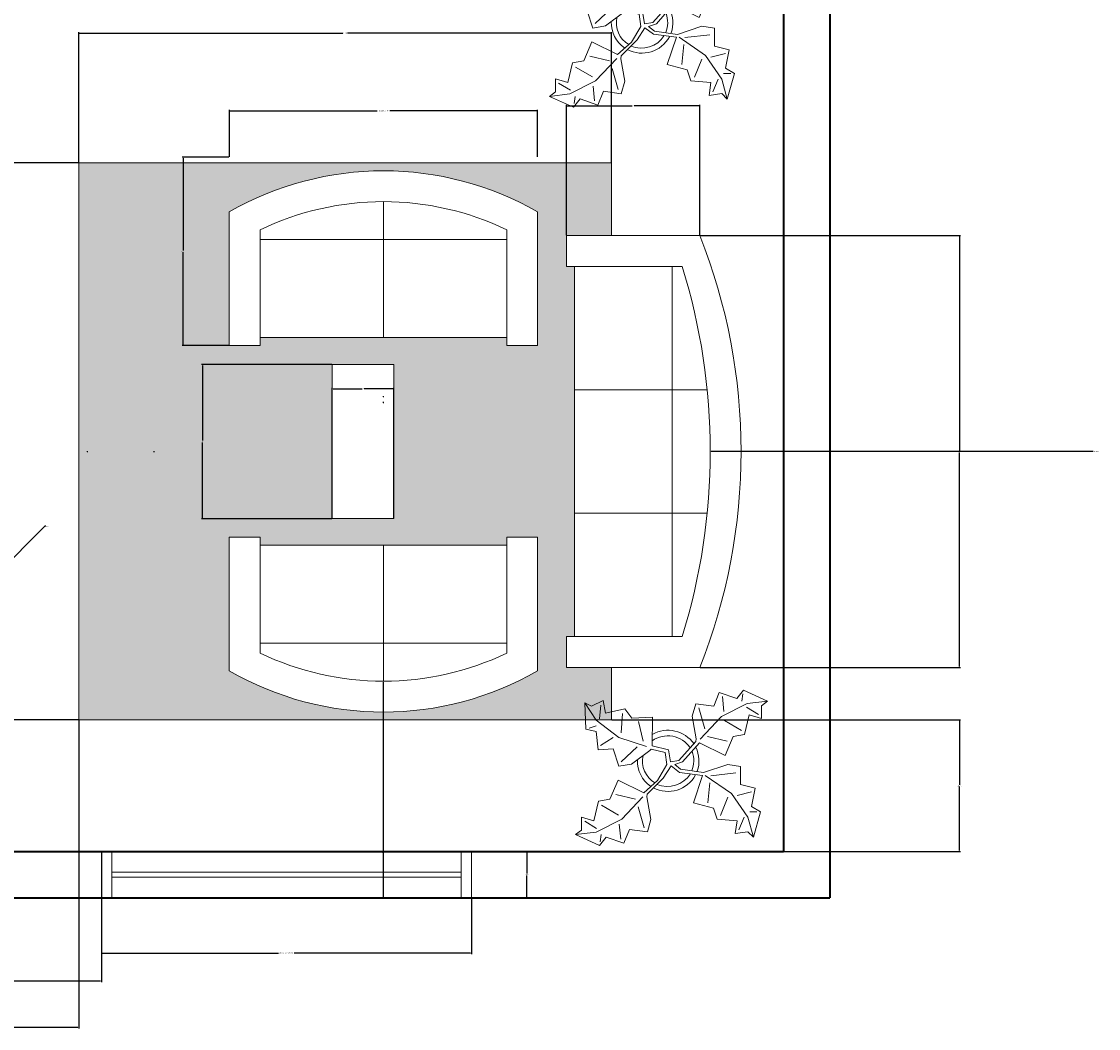
# Model space of a CAD drawing. Units: inches. Extents: x -1 to 436, y -13 to 497.
# Tile 2 of 4: x 227 to 436, y -13 to 183. Entities that reach past the tile are written whole.
import ezdxf

# ---------------------------------------------------------------- set-up
doc = ezdxf.new("R2010")
doc.units = ezdxf.units.IN
for name, color, linetype, lineweight in [('A-ANNO-DIMS', 2, 'Continuous', 18), ('A-FLOR-PATT', 9, 'Continuous', 13), ('A-FURN', 8, 'Continuous', 18), ('A-GLAZ', 4, 'Continuous', 18), ('A-PLNT', 3, 'Continuous', 13), ('A-WALL', 7, 'Continuous', 35)]:
    doc.layers.add(name, color=color, linetype=linetype, lineweight=lineweight)
doc.styles.get("Standard").update_dxf_attribs({"font": 'arial.ttf'})
doc.dimstyles.get("Standard").update_dxf_attribs({"dimtxt": 0.18, "dimasz": 0.18, "dimexe": 0.18, "dimexo": 0.0625, "dimgap": 0.09, "dimtad": 0, "dimtih": 1, "dimtoh": 1, "dimdec": 4, "dimzin": 0, "dimdsep": 46, "dimtxsty": 'Standard', "dimcen": 0.09, "dimadec": 0, "dimazin": 0, "dimtfac": 1, "dimtdec": 4, "dimtofl": 0, "dimtmove": 0, "dimatfit": 3, "dimfxl": 1, "dimtolj": 1, "dimtzin": 0, "dimarcsym": 0})

# ---------------------------------------------------------------- blocks, each defined once
blk = doc.blocks.new('Plant - Rubber or Philodendron')
for p, q in [((8.8871, 10.7908), (9.9809, 13.4933)), ((9.9809, 13.4933), (13.3837, 12.301)), ((10.5828, 12.6946), (10.8893, 9.7953)), ((13.3837, 12.301), (14.68, 13.9039)), ((14.5816, 13.2037), (14.3848, 11.8033)), ((14.68, 13.9039), (19.3848, 11.8146)), ((-16.2005, 11.4774), (-13.9899, 8.1064)), ((-16.2005, 11.4774), (-14.8639, 10.7964)), ((-16.0159, 6.3329), (-16.2005, 11.4774)), ((-14.8639, 10.7964), (-12.6195, 11.8975)), ((-13.3174, 8.325), (-13.0735, 11.0065)), ((-12.6195, 11.8975), (-12.1909, 9.4345)), ((4.6914, 8.8812), (5.3859, 11.2828)), ((5.3859, 11.2828), (8.8871, 10.7908)), ((5.9878, 10.4842), (7.1971, 6.3869)), ((15.3859, 11.3055), (10.3916, 8.7942)), ((15.2875, 10.6053), (17.5907, 9.2105)), ((19.3848, 11.8146), (15.3859, 11.3055)), ((19.3848, 11.8146), (18.1868, 10.9119)), ((18.1868, 10.9119), (18.1925, 8.4119)), ((-12.1909, 9.4345), (-8.3829, 10.3)), ((-8.8369, 9.409), (-9.0894, 5.6095)), ((-8.3829, 10.3), (-7.0549, 8.501)), ((-7.0549, 8.501), (-3.0284, 8.6941)), ((-3.0284, 8.6941), (-3.0709, 3.1041)), ((4.6914, 8.8812), (5.5014, 4.4831)), ((10.3916, 8.7942), (6.2847, 4.4028)), ((15.7909, 9.1065), (14.8995, 5.3044)), ((18.1925, 8.4119), (15.7909, 9.1065)), ((-14.0069, 5.8704), (-16.0159, 6.3329)), ((-15.3434, 6.5514), (-13.9984, 6.9884)), ((-13.9899, 8.1064), (-9.5434, 4.7185)), ((-4.8529, 4.012), (-5.7184, 7.82)), ((14.2977, 6.1031), (10.9934, 7.9956)), ((-13.5868, 2.2894), (-14.0069, 5.8704)), ((-13.1329, 3.1804), (-10.6614, 4.727)), ((-9.5434, 4.7185), (-4.1917, 2.9888)), ((5.4346, 3.9146), (5.5014, 4.4831)), ((7.7005, 4.8881), (11.5025, 3.9967)), ((12.7005, 4.8994), (11.1089, 1.1958)), ((14.8995, 5.3044), (12.7005, 4.8994)), ((-10.6784, 2.491), (-13.5868, 2.2894)), ((-9.5858, -0.8715), (-10.6784, 2.491)), ((-9.1318, 0.0195), (-5.9793, 2.9025)), ((-7.1228, -0.443), (-3.5248, 2.2131)), ((-3.5248, 2.2131), (-3.3011, 2.4355)), ((-3.3011, 2.4355), (-0.5306, 1.7947)), ((-3.0709, 3.1041), (0.0797, 2.3163)), ((0.0797, 2.3163), (0.4866, -0.031)), ((2.1141, 0.2298), (5.4346, 3.9146)), ((6.1032, 3.6844), (2.8262, -0.031)), ((11.1089, 1.1958), (6.1032, 3.6844)), ((-0.5306, 1.7947), (-0.2255, -0.5527)), ((-0.5306, 1.7947), (-0.5306, 1.7947)), ((0.4866, -0.031), (2.1141, 0.2298)), ((-7.1228, -0.443), (-9.5858, -0.8715)), ((-2.019, -3.6148), (-0.2255, -0.5527)), ((-0.9375, -3.1608), (0.5883, -0.8135)), ((0.5883, -0.8135), (2.2447, -2.0916)), ((2.8262, -0.031), (1.3003, -0.5527)), ((1.3003, -0.5527), (2.4193, -1.4655)), ((2.2447, -2.0916), (6.7108, -2.6626)), ((2.4193, -1.4655), (6.895, -2.1175)), ((11.6605, -0.5413), (6.895, -2.1175)), ((11.6605, -0.5413), (14.1354, -0.8948)), ((14.1354, -0.8948), (14.1354, -4.4304)), ((-11.3237, -7.2629), (-9.7321, -3.5593)), ((-9.7321, -3.5593), (-4.7264, -6.0479)), ((-2.019, -3.6148), (-4.7264, -6.0479)), ((-4.0579, -6.2781), (-0.9375, -3.1608)), ((4.943, -7.9659), (6.7108, -2.6626)), ((12.3677, -6.1981), (7.219, -2.6772)), ((8.125, -4.0768), (7.7715, -7.9659)), ((8.3544, -2.7453), (13.1973, -2.1704)), ((-4.1246, -6.8466), (-4.0579, -6.2781)), ((15.5496, -10.7943), (12.3677, -6.1981)), ((16.2567, -5.8446), (13.4283, -6.5517)), ((14.1354, -4.4304), (16.9638, -5.1375)), ((16.9638, -5.1375), (16.2567, -8.673)), ((-14.4141, -11.4699), (-13.5228, -7.6679)), ((-13.5228, -7.6679), (-11.3237, -7.2629)), ((-6.3237, -7.2516), (-10.1257, -6.3602)), ((-9.0148, -11.1577), (-4.9047, -6.8122)), ((-3.3146, -11.2447), (-4.1246, -6.8466)), ((8.8321, -9.0266), (4.943, -7.9659)), ((10.2463, -10.4408), (11.6605, -6.9053)), ((-12.921, -8.4665), (-9.6166, -10.359)), ((-4.611, -12.8477), (-5.8203, -8.7504)), ((9.5392, -11.1479), (8.8321, -9.0266)), ((17.3174, -9.7337), (15.9032, -9.7337)), ((16.2567, -8.673), (18.0245, -9.7337)), ((18.0245, -9.7337), (16.6103, -14.6834)), ((-16.8157, -10.7754), (-14.4141, -11.4699)), ((-16.8101, -13.2754), (-16.8157, -10.7754)), ((-13.9107, -12.9688), (-16.2139, -11.574)), ((-14.0091, -13.669), (-9.0148, -11.1577)), ((-9.206, -15.0581), (-9.5126, -12.1588)), ((-3.3146, -11.2447), (-4.0092, -13.6463)), ((13.4283, -11.5015), (9.5392, -11.1479)), ((13.0748, -13.9763), (13.4283, -11.5015)), ((14.8425, -10.7943), (13.7819, -13.2692)), ((16.6103, -14.6834), (15.5496, -10.7943)), ((-18.008, -14.1781), (-16.8101, -13.2754)), ((-18.008, -14.1781), (-14.0091, -13.669)), ((-13.3032, -16.2674), (-18.008, -14.1781)), ((-12.0069, -14.6645), (-13.3032, -16.2674)), ((-13.2048, -15.5672), (-13.008, -14.1668)), ((-8.6042, -15.8568), (-12.0069, -14.6645)), ((-7.5103, -13.1543), (-8.6042, -15.8568)), ((-4.0092, -13.6463), (-7.5103, -13.1543)), ((15.5496, -13.6228), (13.0748, -13.9763)), ((16.6103, -14.6834), (15.5496, -13.6228))]:
    blk.add_line(p, q)
for centre, radius, start, end in [((0, 0), 6.1275, 34.37569, 120.1028), ((-0.0601, -0.2075), 5.2461, 33.82192, 124.9414), ((-0.098, 0.1364), 6.1288, 341.2017, 26.09184), ((0.0308, 0.1664), 6, 178.6147, 235.1169), ((0.0308, 0.1664), 5, 168.1647, 238.6725), ((-0.2664, 0.1682), 5.2775, 338.4094, 20.03007), ((-0.0234, 0.3825), 6.1492, 242.5812, 331.2714), ((-0.1102, 0.4886), 5.2883, 247.3711, 327.472)]:
    blk.add_arc(centre, radius, start, end)
blk = doc.blocks.new('SOFA-LOVESEAT-60')
for p, q in [((6, 34), (6, 11.47)), ((54, 34), (54, 11.47)), ((54, 32.44), (6, 32.44)), ((30, 32.44), (30, 6)), ((54, 13.38), (6, 13.38))]:
    blk.add_line(p, q)
for points in [[(0, 8), (0, 34), (6, 34)], [(54, 34), (60, 34), (60, 8)]]:
    blk.add_lwpolyline(points)
for centre, radius, start, end in [((30, 61.38), 55.38, 244.3208, 295.6792), ((30, 60.25), 60.25, 240.1371, 299.8628)]:
    blk.add_arc(centre, radius, start, end)
blk = doc.blocks.new('WIN-FIXED-72')
for p, q in [((2, 0), (2, 9)), ((70, 0), (70, 9)), ((2, 5), (70, 5)), ((2, 4), (70, 4))]:
    blk.add_line(p, q)
blk.add_lwpolyline([(0, 9), (72, 9), (72, 0), (0, 0)], close=True)
blk = doc.blocks.new('*D20')
at = {"layer": 'A-ANNO-DIMS', "color": 0, "lineweight": -2, "transparency": 16777216}
for p, q in [((267.14, 156.67), (267.14, 165.79)), ((267.32, 165.61), (295.91, 165.61)), ((326.96, 165.61), (298.36, 165.61)), ((327.14, 156.67), (327.14, 165.79))]:
    blk.add_line(p, q, dxfattribs=at)
at = {"layer": 'A-ANNO-DIMS', "color": 0, "transparency": 16777216}
for points in [[(267.32, 165.64), (267.32, 165.58), (267.14, 165.61)], [(326.96, 165.64), (326.96, 165.58), (327.14, 165.61)]]:
    blk.add_solid(points, dxfattribs=at)
at = {"layer": 'Defpoints', "color": 0, "transparency": 16777216}
for p in [(267.14, 165.61), (267.14, 156.61), (327.14, 156.61)]:
    blk.add_point(p, dxfattribs=at)
at = {"layer": 'A-ANNO-DIMS', "color": 0, "transparency": 16777216, "insert": (297.14, 165.61), "char_height": 0.18, "attachment_point": 5}
blk.add_mtext('\\A1;LOVESEAT 60 TYP.', dxfattribs=at)
blk = doc.blocks.new('*D21')
at = {"layer": 'A-ANNO-DIMS', "color": 0, "lineweight": -2, "transparency": 16777216}
for p, q in [((267.07, 156.61), (257.96, 156.61)), ((258.14, 156.43), (258.14, 138.46)), ((258.14, 120.12), (258.14, 138.09)), ((267.07, 119.94), (257.96, 119.94))]:
    blk.add_line(p, q, dxfattribs=at)
at = {"layer": 'A-ANNO-DIMS', "color": 0, "transparency": 16777216}
for points in [[(258.11, 156.43), (258.17, 156.43), (258.14, 156.61)], [(258.11, 120.12), (258.17, 120.12), (258.14, 119.94)]]:
    blk.add_solid(points, dxfattribs=at)
at = {"layer": 'Defpoints', "color": 0, "transparency": 16777216}
for p in [(267.14, 156.61), (258.14, 119.94), (267.14, 119.94)]:
    blk.add_point(p, dxfattribs=at)
at = {"layer": 'A-ANNO-DIMS', "color": 0, "transparency": 16777216, "insert": (258.14, 138.28), "char_height": 0.18, "attachment_point": 5}
blk.add_mtext('\\A1;37 TYP.', dxfattribs=at)
blk = doc.blocks.new('*D22')
at = {"layer": 'A-ANNO-DIMS', "color": 0, "lineweight": -2, "transparency": 16777216}
for p, q in [((242.25, 12.47), (242.25, 1.55)), ((314.25, 12.47), (314.25, 1.55)), ((242.43, 1.73), (276.74, 1.73)), ((314.07, 1.73), (279.76, 1.73))]:
    blk.add_line(p, q, dxfattribs=at)
at = {"layer": 'A-ANNO-DIMS', "color": 0, "transparency": 16777216}
for points in [[(242.43, 1.76), (242.43, 1.7), (242.25, 1.73)], [(314.07, 1.76), (314.07, 1.7), (314.25, 1.73)]]:
    blk.add_solid(points, dxfattribs=at)
at = {"layer": 'Defpoints', "color": 0, "transparency": 16777216}
for p in [(242.25, 12.53), (314.25, 12.53), (314.25, 1.73)]:
    blk.add_point(p, dxfattribs=at)
at = {"layer": 'A-ANNO-DIMS', "color": 0, "transparency": 16777216, "insert": (278.25, 1.73), "char_height": 0.18, "attachment_point": 5}
blk.add_mtext('\\A1;FIXED WINDOW 72 TYP.', dxfattribs=at)
blk = doc.blocks.new('*D23')
at = {"layer": 'A-ANNO-DIMS', "color": 0, "lineweight": -2, "transparency": 16777216}
for p, q in [((314.31, 21.53), (325.23, 21.53)), ((325.05, 21.35), (325.05, 17.22)), ((325.05, 12.71), (325.05, 16.85)), ((314.31, 12.53), (325.23, 12.53))]:
    blk.add_line(p, q, dxfattribs=at)
at = {"layer": 'A-ANNO-DIMS', "color": 0, "transparency": 16777216}
for points in [[(325.02, 21.35), (325.08, 21.35), (325.05, 21.53)], [(325.02, 12.71), (325.08, 12.71), (325.05, 12.53)]]:
    blk.add_solid(points, dxfattribs=at)
at = {"layer": 'Defpoints', "color": 0, "transparency": 16777216}
for p in [(314.25, 21.53), (325.05, 21.53), (314.25, 12.53)]:
    blk.add_point(p, dxfattribs=at)
at = {"layer": 'A-ANNO-DIMS', "color": 0, "transparency": 16777216, "insert": (325.05, 17.03), "char_height": 0.18, "attachment_point": 5}
blk.add_mtext('\\A1;9 TYP.', dxfattribs=at)
blk = doc.blocks.new('*D30')
at = {"layer": 'A-ANNO-DIMS', "color": 0, "lineweight": -2, "transparency": 16777216}
for p, q in [((181.5, 21.47), (181.5, -3.9)), ((242.25, 21.47), (242.25, -3.9)), ((181.68, -3.72), (211.48, -3.72)), ((242.07, -3.72), (212.27, -3.72))]:
    blk.add_line(p, q, dxfattribs=at)
at = {"layer": 'A-ANNO-DIMS', "color": 0, "transparency": 16777216}
for points in [[(181.68, -3.69), (181.68, -3.75), (181.5, -3.72)], [(242.07, -3.69), (242.07, -3.75), (242.25, -3.72)]]:
    blk.add_solid(points, dxfattribs=at)
at = {"layer": 'Defpoints', "color": 0, "transparency": 16777216}
for p in [(181.5, 21.53), (242.25, 21.53), (181.5, -3.72)]:
    blk.add_point(p, dxfattribs=at)
at = {"layer": 'A-ANNO-DIMS', "color": 0, "transparency": 16777216, "insert": (211.88, -3.72), "char_height": 0.18, "attachment_point": 5}
blk.add_mtext('\\A1;60.75', dxfattribs=at)
blk = doc.blocks.new('*D66')
at = {"layer": 'A-ANNO-DIMS', "color": 0, "lineweight": -2, "transparency": 16777216}
for p, q in [((287.11, 116.27), (261.74, 116.27)), ((261.92, 116.09), (261.92, 101.46)), ((261.92, 86.45), (261.92, 101.09)), ((287.11, 86.27), (261.74, 86.27))]:
    blk.add_line(p, q, dxfattribs=at)
at = {"layer": 'A-ANNO-DIMS', "color": 0, "transparency": 16777216}
for points in [[(261.89, 116.09), (261.95, 116.09), (261.92, 116.27)], [(261.89, 86.45), (261.95, 86.45), (261.92, 86.27)]]:
    blk.add_solid(points, dxfattribs=at)
at = {"layer": 'Defpoints', "color": 0, "transparency": 16777216}
for p in [(261.92, 116.27), (287.17, 116.27), (287.17, 86.27)]:
    blk.add_point(p, dxfattribs=at)
at = {"layer": 'A-ANNO-DIMS', "color": 0, "transparency": 16777216, "insert": (261.92, 101.27), "char_height": 0.18, "attachment_point": 5}
blk.add_mtext('\\A1;30', dxfattribs=at)
blk = doc.blocks.new('*D67')
at = {"layer": 'A-ANNO-DIMS', "color": 0, "lineweight": -2, "transparency": 16777216}
for p, q in [((287.17, 86.34), (287.17, 111.7)), ((287.35, 111.52), (292.97, 111.52)), ((298.99, 111.52), (293.38, 111.52)), ((299.17, 86.34), (299.17, 111.7))]:
    blk.add_line(p, q, dxfattribs=at)
at = {"layer": 'A-ANNO-DIMS', "color": 0, "transparency": 16777216}
for points in [[(287.35, 111.55), (287.35, 111.49), (287.17, 111.52)], [(298.99, 111.55), (298.99, 111.49), (299.17, 111.52)]]:
    blk.add_solid(points, dxfattribs=at)
at = {"layer": 'Defpoints', "color": 0, "transparency": 16777216}
for p in [(299.17, 111.52), (287.17, 86.27), (299.17, 86.27)]:
    blk.add_point(p, dxfattribs=at)
at = {"layer": 'A-ANNO-DIMS', "color": 0, "transparency": 16777216, "insert": (293.17, 111.52), "char_height": 0.18, "attachment_point": 5}
blk.add_mtext('\\A1;12', dxfattribs=at)
blk = doc.blocks.new('*D68')
at = {"layer": 'A-ANNO-DIMS', "color": 0, "lineweight": -2, "transparency": 16777216}
for p, q in [((358.8, 141.33), (409.43, 141.33)), ((409.25, 141.15), (409.25, 99.51)), ((409.25, 57.51), (409.25, 99.15)), ((358.8, 57.33), (409.43, 57.33))]:
    blk.add_line(p, q, dxfattribs=at)
at = {"layer": 'A-ANNO-DIMS', "color": 0, "transparency": 16777216}
for points in [[(409.22, 141.15), (409.28, 141.15), (409.25, 141.33)], [(409.22, 57.51), (409.28, 57.51), (409.25, 57.33)]]:
    blk.add_solid(points, dxfattribs=at)
at = {"layer": 'Defpoints', "color": 0, "transparency": 16777216}
for p in [(358.74, 141.33), (358.74, 57.33), (409.25, 57.33)]:
    blk.add_point(p, dxfattribs=at)
at = {"layer": 'A-ANNO-DIMS', "color": 0, "transparency": 16777216, "insert": (409.25, 99.33), "char_height": 0.18, "attachment_point": 5}
blk.add_mtext('\\A1;84', dxfattribs=at)
blk = doc.blocks.new('*D69')
at = {"layer": 'A-ANNO-DIMS', "color": 0, "lineweight": -2, "transparency": 16777216}
for p, q in [((332.74, 141.39), (332.74, 166.76)), ((332.92, 166.58), (345.51, 166.58)), ((358.56, 166.58), (345.96, 166.58)), ((358.74, 141.39), (358.74, 166.76))]:
    blk.add_line(p, q, dxfattribs=at)
at = {"layer": 'A-ANNO-DIMS', "color": 0, "transparency": 16777216}
for points in [[(332.92, 166.61), (332.92, 166.55), (332.74, 166.58)], [(358.56, 166.61), (358.56, 166.55), (358.74, 166.58)]]:
    blk.add_solid(points, dxfattribs=at)
at = {"layer": 'Defpoints', "color": 0, "transparency": 16777216}
for p in [(358.74, 166.58), (332.74, 141.33), (358.74, 141.33)]:
    blk.add_point(p, dxfattribs=at)
at = {"layer": 'A-ANNO-DIMS', "color": 0, "transparency": 16777216, "insert": (345.74, 166.58), "char_height": 0.18, "attachment_point": 5}
blk.add_mtext('\\A1;26', dxfattribs=at)
blk = doc.blocks.new('*D70')
at = {"layer": 'A-ANNO-DIMS', "color": 0, "lineweight": -2, "transparency": 16777216}
for p, q in [((237.77, 155.49), (212.4, 155.49)), ((212.58, 155.31), (212.58, 101.48)), ((212.58, 47.29), (212.58, 101.11)), ((237.77, 47.11), (212.4, 47.11))]:
    blk.add_line(p, q, dxfattribs=at)
at = {"layer": 'A-ANNO-DIMS', "color": 0, "transparency": 16777216}
for points in [[(212.55, 155.31), (212.61, 155.31), (212.58, 155.49)], [(212.55, 47.29), (212.61, 47.29), (212.58, 47.11)]]:
    blk.add_solid(points, dxfattribs=at)
at = {"layer": 'Defpoints', "color": 0, "transparency": 16777216}
for p in [(212.58, 155.49), (237.83, 155.49), (237.83, 47.11)]:
    blk.add_point(p, dxfattribs=at)
at = {"layer": 'A-ANNO-DIMS', "color": 0, "transparency": 16777216, "insert": (212.58, 101.3), "char_height": 0.18, "attachment_point": 5}
blk.add_mtext('\\A1;108.38', dxfattribs=at)
blk = doc.blocks.new('*D71')
at = {"layer": 'A-ANNO-DIMS', "color": 0, "lineweight": -2, "transparency": 16777216}
for p, q in [((237.83, 155.55), (237.83, 180.92)), ((238.01, 180.74), (289.21, 180.74)), ((341.33, 180.74), (290.12, 180.74)), ((341.51, 155.55), (341.51, 180.92))]:
    blk.add_line(p, q, dxfattribs=at)
at = {"layer": 'A-ANNO-DIMS', "color": 0, "transparency": 16777216}
for points in [[(238.01, 180.77), (238.01, 180.71), (237.83, 180.74)], [(341.33, 180.77), (341.33, 180.71), (341.51, 180.74)]]:
    blk.add_solid(points, dxfattribs=at)
at = {"layer": 'Defpoints', "color": 0, "transparency": 16777216}
for p in [(341.51, 180.74), (237.83, 155.49), (341.51, 155.49)]:
    blk.add_point(p, dxfattribs=at)
at = {"layer": 'A-ANNO-DIMS', "color": 0, "transparency": 16777216, "insert": (289.67, 180.74), "char_height": 0.18, "attachment_point": 5}
blk.add_mtext('\\A1;103.68', dxfattribs=at)
blk = doc.blocks.new('*D72')
at = {"layer": 'A-ANNO-DIMS', "color": 0, "lineweight": -2, "transparency": 16777216}
for p, q in [((237.83, 229.51), (212.46, 229.53)), ((212.64, 229.35), (212.61, 192.7)), ((212.58, 155.69), (212.61, 192.34)), ((237.77, 155.49), (212.4, 155.51))]:
    blk.add_line(p, q, dxfattribs=at)
at = {"layer": 'A-ANNO-DIMS', "color": 0, "transparency": 16777216}
for points in [[(212.61, 229.35), (212.67, 229.35), (212.64, 229.53)], [(212.55, 155.69), (212.61, 155.69), (212.58, 155.51)]]:
    blk.add_solid(points, dxfattribs=at)
at = {"layer": 'Defpoints', "color": 0, "transparency": 16777216}
for p in [(212.64, 229.53), (237.89, 229.51), (237.83, 155.49)]:
    blk.add_point(p, dxfattribs=at)
at = {"layer": 'A-ANNO-DIMS', "color": 0, "transparency": 16777216, "insert": (212.61, 192.52), "char_height": 0.18, "attachment_point": 5}
blk.add_mtext('\\A1;74.03', dxfattribs=at)
blk = doc.blocks.new('*D76')
at = {"layer": 'A-ANNO-DIMS', "color": 0, "lineweight": -2, "transparency": 16777216}
for p, q in [((341.57, 47.11), (409.43, 47.11)), ((409.25, 46.93), (409.25, 34.5)), ((409.25, 21.71), (409.25, 34.14)), ((375.06, 21.53), (409.43, 21.53))]:
    blk.add_line(p, q, dxfattribs=at)
at = {"layer": 'A-ANNO-DIMS', "color": 0, "transparency": 16777216}
for points in [[(409.22, 46.93), (409.28, 46.93), (409.25, 47.11)], [(409.22, 21.71), (409.28, 21.71), (409.25, 21.53)]]:
    blk.add_solid(points, dxfattribs=at)
at = {"layer": 'Defpoints', "color": 0, "transparency": 16777216}
for p in [(341.51, 47.11), (409.25, 47.11), (375, 21.53)]:
    blk.add_point(p, dxfattribs=at)
at = {"layer": 'A-ANNO-DIMS', "color": 0, "transparency": 16777216, "insert": (409.25, 34.32), "char_height": 0.18, "attachment_point": 5}
blk.add_mtext('\\A1;25.573', dxfattribs=at)
blk = doc.blocks.new('*D77')
at = {"layer": 'A-ANNO-DIMS', "color": 0, "lineweight": -2, "transparency": 16777216}
for p, q in [((237.83, 47.04), (237.83, -12.9)), ((181.5, 21.47), (181.5, -12.9)), ((181.68, -12.72), (209.27, -12.72)), ((237.65, -12.72), (210.06, -12.72))]:
    blk.add_line(p, q, dxfattribs=at)
at = {"layer": 'A-ANNO-DIMS', "color": 0, "transparency": 16777216}
for points in [[(181.68, -12.69), (181.68, -12.75), (181.5, -12.72)], [(237.65, -12.69), (237.65, -12.75), (237.83, -12.72)]]:
    blk.add_solid(points, dxfattribs=at)
at = {"layer": 'Defpoints', "color": 0, "transparency": 16777216}
for p in [(237.83, 47.11), (181.5, 21.53), (237.83, -12.72)]:
    blk.add_point(p, dxfattribs=at)
at = {"layer": 'A-ANNO-DIMS', "color": 0, "transparency": 16777216, "insert": (209.67, -12.72), "char_height": 0.18, "attachment_point": 5}
blk.add_mtext('\\A1;56.33', dxfattribs=at)
blk = doc.blocks.new('*D78')
at = {"layer": 'A-ANNO-DIMS', "color": 0, "lineweight": -2, "transparency": 16777216}
for p, q in [((252.4, 99.33), (252.58, 99.33)), ((252.49, 99.24), (252.49, 99.42)), ((435.29, 99.33), (366.92, 99.33))]:
    blk.add_line(p, q, dxfattribs=at)
at = {"layer": 'A-ANNO-DIMS', "color": 0, "transparency": 16777216}
blk.add_solid([(366.92, 99.36), (366.92, 99.3), (366.74, 99.33)], dxfattribs=at)
at = {"layer": 'Defpoints', "color": 0, "transparency": 16777216}
for p in [(252.49, 99.33), (366.74, 99.33)]:
    blk.add_point(p, dxfattribs=at)
at = {"layer": 'A-ANNO-DIMS', "color": 0, "transparency": 16777216, "insert": (435.84, 99.33), "char_height": 0.18, "attachment_point": 5}
blk.add_mtext('\\A1;R114.25', dxfattribs=at)
blk = doc.blocks.new('*D79')
at = {"layer": 'A-ANNO-DIMS', "color": 0, "lineweight": -2, "transparency": 16777216}
for p, q in [((239.45, 99.33), (239.63, 99.33)), ((239.54, 99.24), (239.54, 99.42)), ((433.45, 99.33), (360.92, 99.33))]:
    blk.add_line(p, q, dxfattribs=at)
at = {"layer": 'A-ANNO-DIMS', "color": 0, "transparency": 16777216}
blk.add_solid([(360.92, 99.36), (360.92, 99.3), (360.74, 99.33)], dxfattribs=at)
at = {"layer": 'Defpoints', "color": 0, "transparency": 16777216}
for p in [(239.54, 99.33), (360.74, 99.33)]:
    blk.add_point(p, dxfattribs=at)
at = {"layer": 'A-ANNO-DIMS', "color": 0, "transparency": 16777216, "insert": (433.93, 99.33), "char_height": 0.18, "attachment_point": 5}
blk.add_mtext('\\A1;R121.2', dxfattribs=at)
blk = doc.blocks.new('*D80')
at = {"layer": 'A-ANNO-DIMS', "color": 0, "lineweight": -2, "transparency": 16777216}
for p, q in [((297.14, 108.81), (297.14, 108.99)), ((297.05, 108.9), (297.23, 108.9)), ((297.13, 12.5), (297.13, 48.47)), ((296.95, 12.5), (297.13, 12.5))]:
    blk.add_line(p, q, dxfattribs=at)
at = {"layer": 'A-ANNO-DIMS', "color": 0, "transparency": 16777216}
blk.add_solid([(297.1, 48.47), (297.16, 48.47), (297.13, 48.65)], dxfattribs=at)
at = {"layer": 'Defpoints', "color": 0, "transparency": 16777216}
for p in [(297.14, 108.9), (297.13, 48.65)]:
    blk.add_point(p, dxfattribs=at)
at = {"layer": 'A-ANNO-DIMS', "color": 0, "transparency": 16777216, "insert": (296.28, 12.5), "char_height": 0.18, "attachment_point": 5}
blk.add_mtext('\\A1;2X R60.25', dxfattribs=at)
blk = doc.blocks.new('*D81')
at = {"layer": 'A-ANNO-DIMS', "color": 0, "lineweight": -2, "transparency": 16777216}
for p, q in [((297.05, 110.04), (297.23, 110.04)), ((297.14, 109.95), (297.14, 110.13)), ((297.13, 21.42), (297.13, 54.47)), ((296.95, 21.42), (297.13, 21.42))]:
    blk.add_line(p, q, dxfattribs=at)
at = {"layer": 'A-ANNO-DIMS', "color": 0, "transparency": 16777216}
blk.add_solid([(297.1, 54.47), (297.16, 54.47), (297.13, 54.65)], dxfattribs=at)
at = {"layer": 'Defpoints', "color": 0, "transparency": 16777216}
for p in [(297.14, 110.04), (297.13, 54.65)]:
    blk.add_point(p, dxfattribs=at)
at = {"layer": 'A-ANNO-DIMS', "color": 0, "transparency": 16777216, "insert": (296.28, 21.42), "char_height": 0.18, "attachment_point": 5}
blk.add_mtext('\\A1;2X R55.38', dxfattribs=at)
blk = doc.blocks.new('*D83')
at = {"layer": 'A-ANNO-DIMS', "color": 0, "lineweight": -2, "transparency": 16777216}
for p, q in [((231.24, 84.78), (211.22, 64.75)), ((231.42, 84.78), (231.24, 84.78)), ((177.41, 31.03), (177.59, 31.03)), ((177.5, 30.94), (177.5, 31.12))]:
    blk.add_line(p, q, dxfattribs=at)
at = {"layer": 'A-ANNO-DIMS', "color": 0, "transparency": 16777216}
blk.add_solid([(211.2, 64.77), (211.24, 64.73), (211.09, 64.62)], dxfattribs=at)
at = {"layer": 'Defpoints', "color": 0, "transparency": 16777216}
for p in [(211.09, 64.62), (177.5, 31.03)]:
    blk.add_point(p, dxfattribs=at)
at = {"layer": 'A-ANNO-DIMS', "color": 0, "transparency": 16777216, "insert": (231.83, 84.78), "char_height": 0.18, "attachment_point": 5}
blk.add_mtext('\\A1;R47.5', dxfattribs=at)

msp = doc.modelspace()

# ---------------------------------------------------------------- hatches: boundary and pattern name
at = {"layer": 'A-FLOR-PATT'}
h = msp.add_hatch(color=256, dxfattribs=at)
h.dxf.hatch_style = 1
h.paths.add_polyline_path([(334.2932, 135.3315), (332.7353, 135.3315), (332.7353, 141.3315), (341.5066, 141.3315), (341.5066, 155.4864), (237.8302, 155.4864), (237.8302, 47.1064), (341.5066, 47.1064), (341.5066, 57.3315), (332.7353, 57.3315), (332.7353, 63.3315), (334.2932, 63.3315)])
h.paths.add_polyline_path([(321.1354, 119.9418), (321.1354, 121.4998), (273.1354, 121.4998), (273.1354, 119.9418), (267.1354, 119.9418), (267.1354, 145.9417, -0.26666697), (327.1354, 145.9417), (327.1354, 119.9418)], flags=16)
h.paths.add_polyline_path([(299.175, 86.2737), (287.175, 86.2737), (287.175, 116.2737), (299.175, 116.2737)], flags=16)
h.paths.add_polyline_path([(321.1354, 82.6511), (327.1354, 82.6511), (327.1354, 56.6511, -0.26666697), (267.1354, 56.6511), (267.1354, 82.6511), (273.1354, 82.6511), (273.1354, 81.0931), (321.1354, 81.0931)], flags=16)

# ---------------------------------------------------------------- linework, layer by layer
at = {"layer": 'A-FURN'}
for p, q in [((237.8302, 155.4864), (341.5066, 155.4864)), ((237.8302, 47.1064), (237.8302, 155.4864)), ((341.5066, 155.4864), (341.5066, 141.3315)), ((332.7353, 135.3315), (355.2657, 135.3315)), ((334.2932, 135.3315), (334.2932, 63.3315)), ((353.3534, 135.3313), (353.3534, 63.3317)), ((299.175, 116.2737), (287.175, 116.2737)), ((287.175, 116.2737), (287.175, 86.2737)), ((299.175, 86.2737), (299.175, 116.2737)), ((334.2932, 111.3315), (360.1382, 111.3315)), ((287.175, 86.2737), (299.175, 86.2737)), ((334.2932, 87.3315), (360.1382, 87.3315)), ((332.7353, 63.3315), (355.2657, 63.3315)), ((341.5066, 57.3315), (341.5066, 47.1064)), ((341.5066, 47.1064), (237.8302, 47.1064))]:
    msp.add_line(p, q, dxfattribs=at)
for points in [[(332.7353, 135.3315), (332.7353, 141.3315), (358.7353, 141.3315)], [(358.7353, 57.3315), (332.7353, 57.3315), (332.7353, 63.3315)]]:
    msp.add_lwpolyline(points, dxfattribs=at)
for centre, radius, start, end in [((252.4853, 99.3315), 114.25, 338.43141, 21.5686), ((239.5385, 99.3315), 121.1968, 342.72033, 17.2797)]:
    msp.add_arc(centre, radius, start, end, dxfattribs=at)
at = {"layer": 'A-WALL'}
for p, q in [((384, 471.5331), (384, 12.5331)), ((375, 390.5331), (375, 21.5331)), ((181.5, 21.5331), (375, 21.5331)), ((177, 12.5331), (384, 12.5331))]:
    msp.add_line(p, q, dxfattribs=at)

# ---------------------------------------------------------------- block references
at = {"layer": 'A-FURN', "rotation": 180.0000448048175}
msp.add_blockref('SOFA-LOVESEAT-60', (327.1358, 153.9419), dxfattribs=at)
at = {"layer": 'A-FURN'}
msp.add_blockref('SOFA-LOVESEAT-60', (267.135, 48.651), dxfattribs=at)
at = {"layer": 'A-GLAZ'}
msp.add_blockref('WIN-FIXED-72', (242.25, 12.533), dxfattribs=at)
at = {"layer": 'A-PLNT'}
for p in [(347.4393, 182.5896), (352.5154, 38.9808)]:
    msp.add_blockref('Plant - Rubber or Philodendron', p, dxfattribs=at)

# ---------------------------------------------------------------- dimensions: what is measured, and where the dimension line sits
at = {"layer": 'A-ANNO-DIMS'}
for base, p1, p2, angle, override, picture, middle in [((212.6448, 229.5338), (237.8302, 155.4864), (237.8948, 229.5117), 89.949986, {"dimdec": 2, "dimlfac": 1, "dimrnd": 0, "dimzin": 0, "dimdsep": 46, "dimlunit": 2}, '*D72', (212.6125, 192.5211)), ((358.7353, 166.5815), (332.7353, 141.3315), (358.7353, 141.3315), 359.999958, {"dimdec": 0, "dimlfac": 1, "dimrnd": 0, "dimzin": 0, "dimdsep": 46, "dimlunit": 2}, '*D69', (345.7353, 166.5815)), ((212.5802, 155.4864), (237.8302, 47.1064), (237.8302, 155.4864), 90, {"dimdec": 2, "dimlfac": 1, "dimrnd": 0, "dimzin": 0, "dimdsep": 46, "dimlunit": 2}, '*D70', (212.5802, 101.2964)), ((409.25, 57.3315), (358.7353, 141.3315), (358.7353, 57.3315), 90, {"dimdec": 0, "dimlfac": 1, "dimrnd": 0, "dimzin": 0, "dimdsep": 46, "dimlunit": 2}, '*D68', (409.25, 99.3315)), ((261.925, 116.2737), (287.175, 86.2737), (287.175, 116.2737), 90, {"dimdec": 0, "dimlfac": 1, "dimrnd": 0, "dimzin": 0, "dimdsep": 46, "dimlunit": 2}, '*D66', (261.925, 101.2737)), ((409.25, 47.1064), (375, 21.5331), (341.5066, 47.1064), 90, {"dimdec": 3, "dimlfac": 1, "dimrnd": 0, "dimzin": 0, "dimdsep": 46, "dimlunit": 2}, '*D76', (409.25, 34.3198)), ((181.5, -3.7169), (242.25, 21.5331), (181.5, 21.5331), 180, {"dimdec": 2, "dimlfac": 1, "dimrnd": 0, "dimzin": 0, "dimdsep": 46, "dimlunit": 2}, '*D30', (211.875, -3.7169))]:
    dim = msp.add_linear_dim(base=base, p1=p1, p2=p2, angle=angle, dimstyle='Standard', override=override, dxfattribs=at)
    dim.commit()
    dim.dimension.update_dxf_attribs({"geometry": picture, "text_midpoint": middle})
for base, p1, p2, override, picture, middle in [((341.5066, 180.7364), (237.8302, 155.4864), (341.5066, 155.4864), {"dimdec": 2, "dimlfac": 1, "dimrnd": 0, "dimzin": 0, "dimdsep": 46, "dimlunit": 2}, '*D71', (289.6684, 180.7364)), ((299.175, 111.5237), (287.175, 86.2737), (299.175, 86.2737), {"dimdec": 0, "dimlfac": 1, "dimrnd": 0, "dimzin": 0, "dimdsep": 46, "dimlunit": 2}, '*D67', (293.175, 111.5237)), ((237.8302, -12.7169), (181.5, 21.5331), (237.8302, 47.1064), {"dimdec": 2, "dimlfac": 1, "dimrnd": 0, "dimzin": 0, "dimdsep": 46, "dimlunit": 2}, '*D77', (209.6651, -12.7169))]:
    dim = msp.add_linear_dim(base=base, p1=p1, p2=p2, dimstyle='Standard', override=override, dxfattribs=at)
    dim.commit()
    dim.dimension.update_dxf_attribs({"geometry": picture, "text_midpoint": middle})
for base, p1, p2, angle, text, picture, middle in [((267.1354, 165.6084), (327.1354, 156.6084), (267.1354, 156.6084), 180.000045, 'LOVESEAT <> TYP.', '*D20', (297.1354, 165.6084)), ((258.1354, 119.9417), (267.1354, 156.6084), (267.1354, 119.9417), 270.000045, '<> TYP.', '*D21', (258.1354, 138.2751)), ((325.05, 21.5331), (314.25, 12.5331), (314.25, 21.5331), 90, '<> TYP.', '*D23', (325.05, 17.0331))]:
    dim = msp.add_linear_dim(base=base, p1=p1, p2=p2, angle=angle, text=text, dimstyle='Standard', override={"dimdec": 0, "dimlfac": 1, "dimrnd": 0, "dimzin": 0, "dimdsep": 46, "dimlunit": 2}, dxfattribs=at)
    dim.commit()
    dim.dimension.update_dxf_attribs({"geometry": picture, "text_midpoint": middle})
for center, mpoint, picture, middle in [((297.1354, 108.9011), (297.135, 48.6511), '*D80', (296.2793, 12.5011)), ((297.1354, 110.0355), (297.135, 54.651), '*D81', (296.2798, 21.4204))]:
    dim = msp.add_radius_dim(center=center, mpoint=mpoint, text='2X <>', dimstyle='Standard', override={"dimdec": 2, "dimlfac": 1, "dimrnd": 0, "dimzin": 0, "dimdsep": 46, "dimlunit": 2}, dxfattribs=at)
    dim.commit()
    dim.dimension.update_dxf_attribs({"geometry": picture, "text_midpoint": middle, "dimtype": 164})
for center, mpoint, override, picture, middle in [((239.5385, 99.3315), (360.7353, 99.331), {"dimdec": 1, "dimlfac": 1, "dimrnd": 0, "dimzin": 0, "dimdsep": 46, "dimlunit": 2}, '*D79', (433.4534, 99.3307)), ((252.4853, 99.3315), (366.7353, 99.331), {"dimdec": 2, "dimlfac": 1, "dimrnd": 0, "dimzin": 0, "dimdsep": 46, "dimlunit": 2}, '*D78', (435.2853, 99.3307)), ((177.5, 31.0331), (211.089, 64.623), {"dimdec": 1, "dimlfac": 1, "dimrnd": 0, "dimzin": 0, "dimdsep": 46, "dimlunit": 2}, '*D83', (231.833, 84.7769))]:
    dim = msp.add_radius_dim(center=center, mpoint=mpoint, dimstyle='Standard', override=override, dxfattribs=at)
    dim.commit()
    dim.dimension.update_dxf_attribs({"geometry": picture, "text_midpoint": middle, "dimtype": 164})
dim = msp.add_linear_dim(base=(314.25, 1.7331), p1=(242.25, 12.5331), p2=(314.25, 12.5331), text='FIXED WINDOW <> TYP.', dimstyle='Standard', override={"dimdec": 0, "dimlfac": 1, "dimrnd": 0, "dimzin": 0, "dimdsep": 46, "dimlunit": 2}, dxfattribs=at)
dim.commit()
dim.dimension.update_dxf_attribs({"geometry": '*D22', "text_midpoint": (278.25, 1.7331)})

doc.saveas('drawing.dxf')
